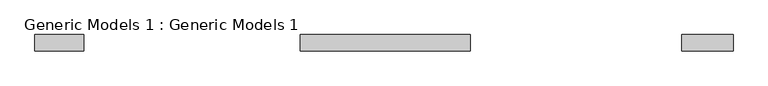
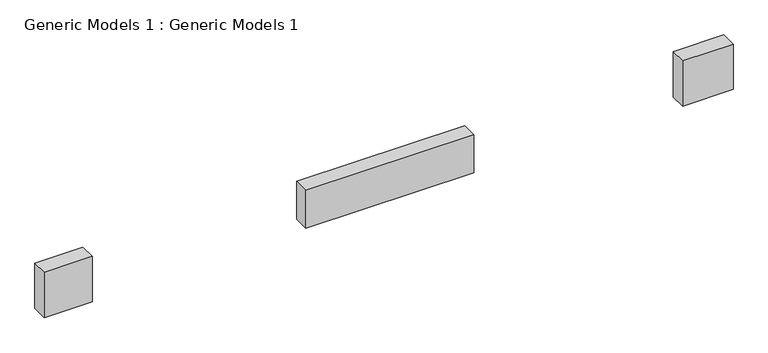
"""IFC4 building model written with IfcOpenShell, lengths in millimetres: proxy geometry, Generic Models 1 : Generic Models 1."""

from ifc_helpers import new_model, si_unit, frame, origin, place, context, project, spatial, polyline, outline, extrude, source, transform, mapped, element, save


def generic_models_1_generic_models_1_6252d277(model_context):
    return source(origin(), model_context, "Body", "SweptSolid", [
        extrude(outline(polyline([(-6191.9640964, -3218.996468), (-7106.3640964, -3218.996468), (-7106.3640964, -2914.196468), (-6191.9640964, -2914.196468), (-6191.9640964, -3218.996468)])), frame((0.0, 0.0, 9741.5274693), z_axis=(0.0, 0.0, 1.0), x_axis=(1.0, 0.0, 0.0)), (0.0, 0.0, 1.0), 914.4),
        extrude(outline(polyline([(6015.9109036, -3218.996468), (5053.7726186, -3218.996468), (5053.7726186, -2914.196468), (6015.9109036, -2914.196468), (6015.9109036, -3218.996468)])), frame((0.0, 0.0, 9741.5274693), z_axis=(0.0, 0.0, 1.0), x_axis=(1.0, 0.0, 0.0)), (0.0, 0.0, 1.0), 914.4),
        extrude(outline(polyline([(1078.0462838, -3218.996468), (-2122.3537162, -3218.996468), (-2122.3537162, -2914.196468), (1078.0462838, -2914.196468), (1078.0462838, -3218.996468)])), frame((0.0, 0.0, 9795.4996766), z_axis=(0.0, 0.0, 1.0), x_axis=(1.0, 0.0, 0.0)), (0.0, 0.0, 1.0), 762.0),
    ])


if __name__ == "__main__":
    model = new_model("IFC4")
    model_context = context("Model", 3, world=origin())
    ifc_project = project(units=[si_unit("LENGTHUNIT", "METRE", prefix="MILLI")], contexts=[model_context])
    site = spatial("IfcSite", under=ifc_project)
    building = spatial("IfcBuilding", under=site)
    placement = place(None, origin())
    generic_models_1_generic_models_1_shape = generic_models_1_generic_models_1_6252d277(model_context)
    element("IfcBuildingElementProxy", 1, Name="Generic Models 1 : Generic Models 1", ObjectType="Generic Models 1 : Generic Models 1", at=placement, inside=building, context=model_context, shape_type="MappedRepresentation", body=[
        mapped(generic_models_1_generic_models_1_shape, transform((0.0, 0.0, 0.0), x_axis=(1.0, 0.0, 0.0), y_axis=(0.0, 1.0, 0.0), z_axis=(0.0, 0.0, 1.0))),
    ])
    save(model, "model.ifc")

# Revit data of these elements
# Element 1 (IfcBuildingElementProxy, "Generic Models 1 : Generic Models 1")
#   Materials on its faces: "Parking Stripe", "Carpet (1)"
# Materials
#   "Parking Stripe": class "Paint", colour RGB 250 250 91, transparency 0, Cost = 0
#   "Carpet (1)": class "Carpet", colour RGB 124 80 67, transparency 0, Description = "Interior finish", Cost = 0
